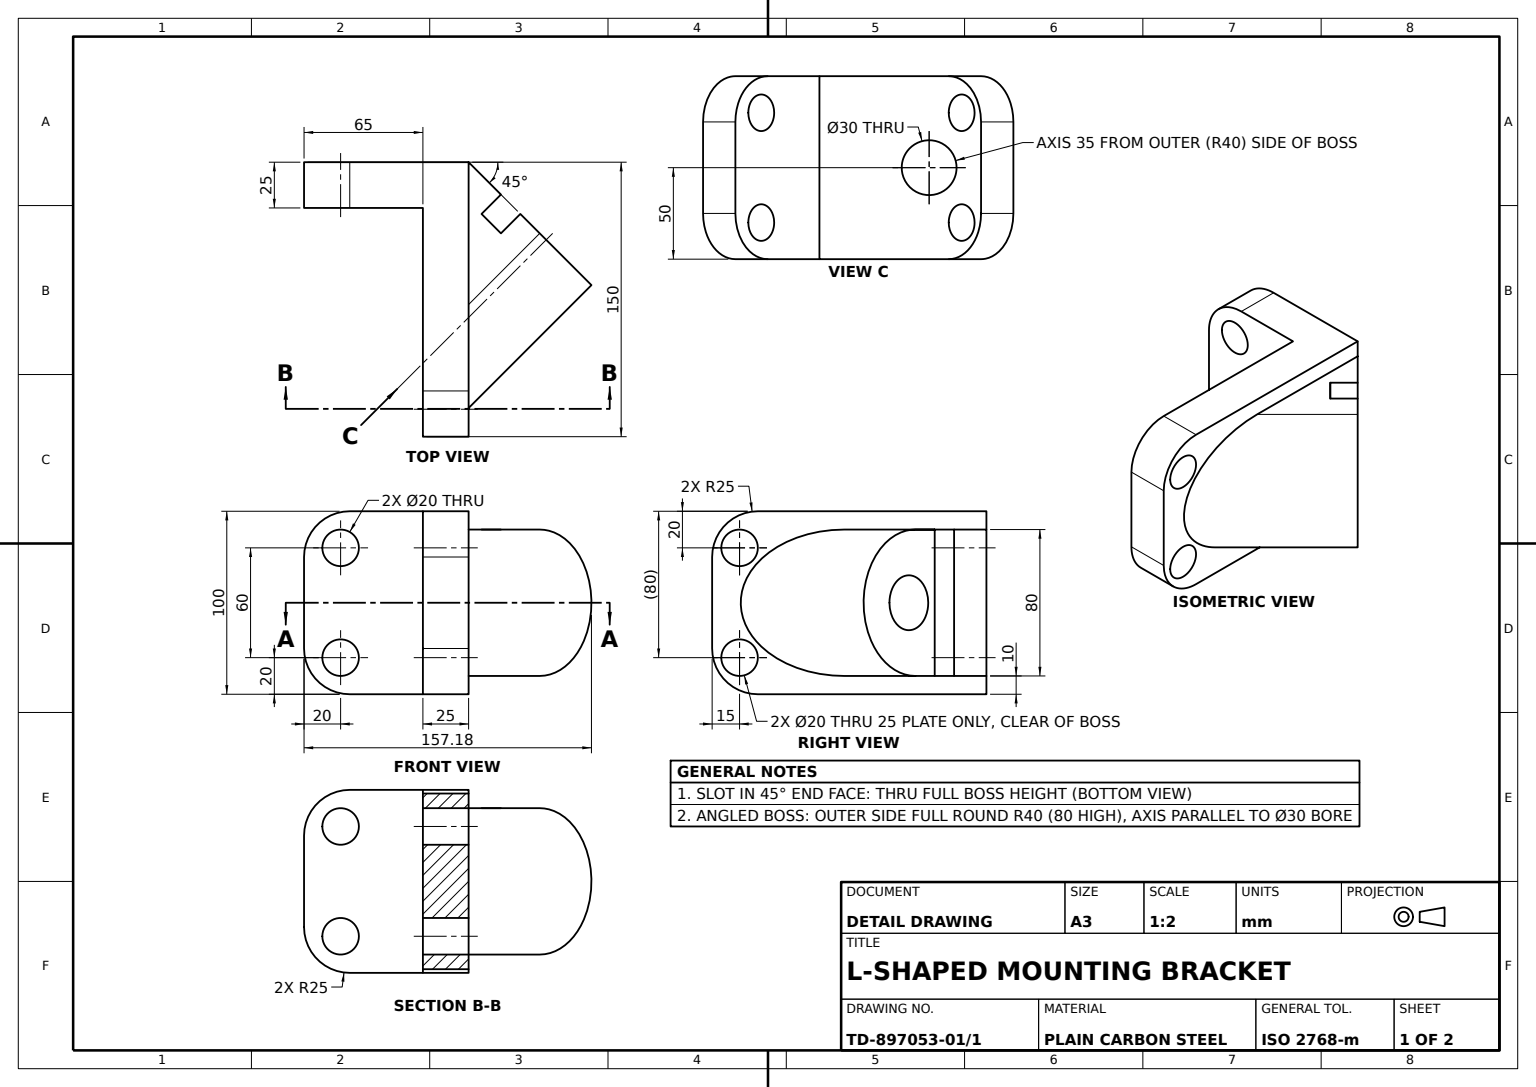
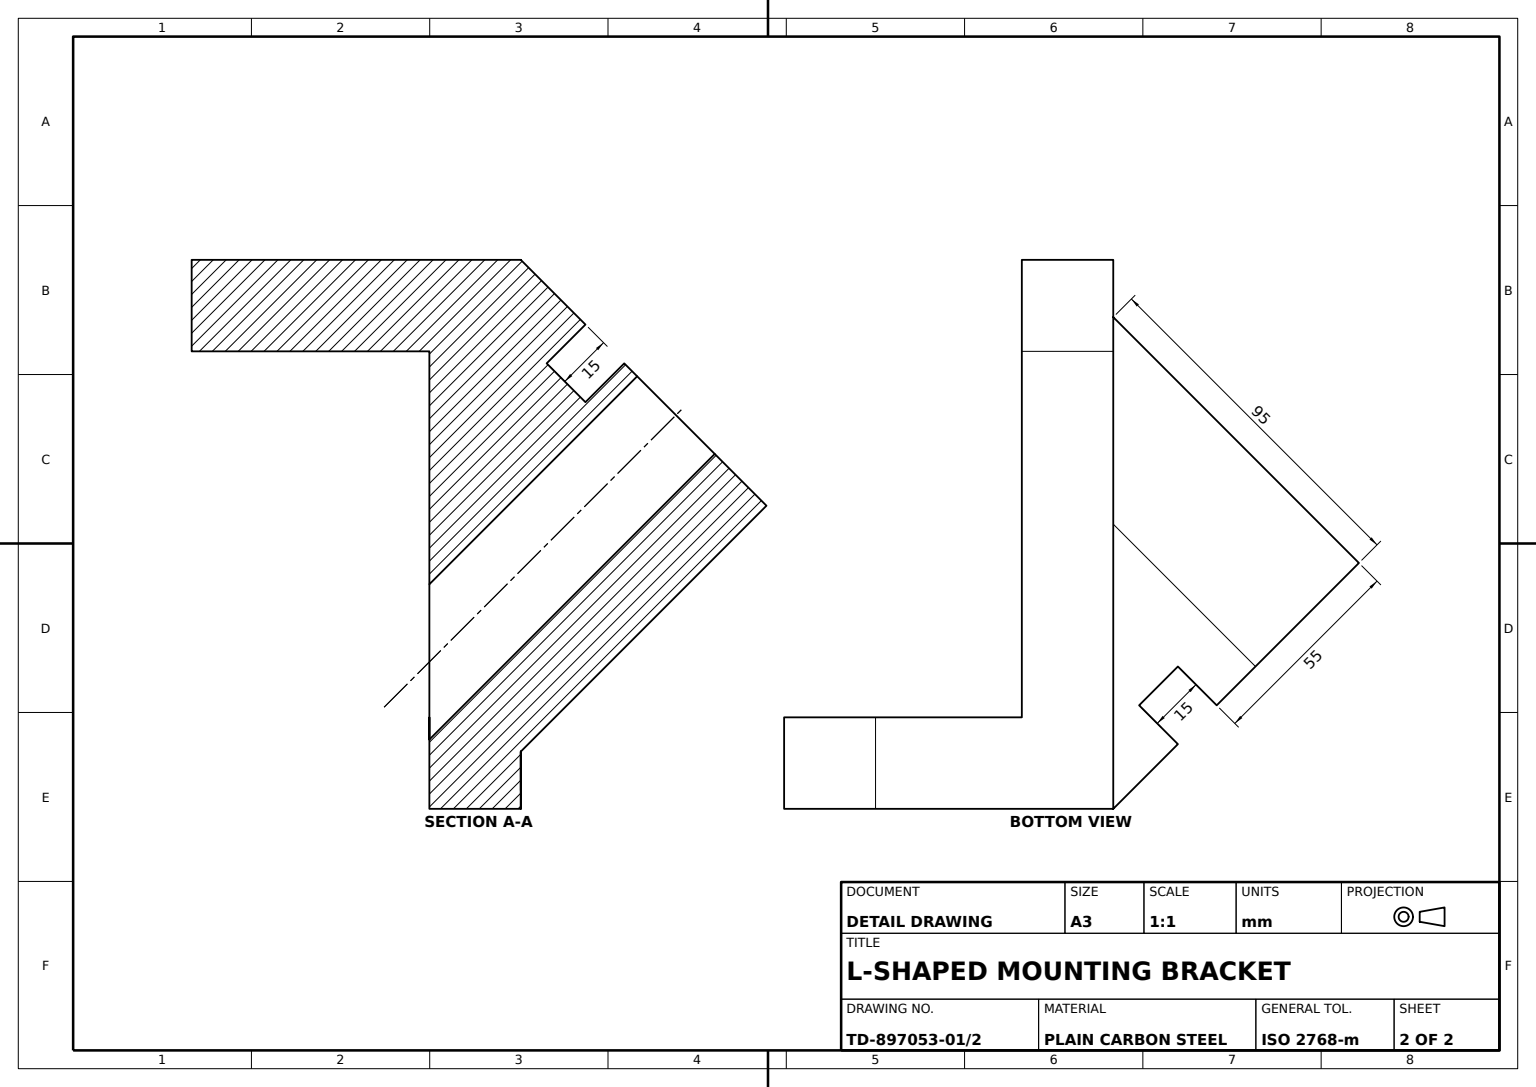
from build123d import *

# Parameters (mm, degrees)
BASE_PLATE_SKETCH_W           = 150
BASE_PLATE_SKETCH_H           = 100
BASE_PLATE_150X100X25_DEPTH   = 25
UPRIGHT_PLATE_SKETCH_W        = 25
UPRIGHT_PLATE_SKETCH_H        = 100
UPRIGHT_PLATE_DEPTH           = 65
ANGLED_BOSS_REACH             = 179.236
BOSS_SLOT_REACH               = 149.733
BOSS_BORE_REACH               = 179.236
BOSS_BORE_SKETCH_R            = 15
BASE_PLATE_HOLES_REACH        = 129.377
BASE_PLATE_HOLES_SKETCH_R     = 10
UPRIGHT_PLATE_HOLES_REACH     = 183.934
UPRIGHT_PLATE_HOLES_SKETCH_R  = 10
UPRIGHT_CORNER_FILLET_R25_A_R = 25
UPRIGHT_CORNER_FILLET_R25_B_R = 25
BASE_CORNER_FILLET_R25_A_R    = 25
BASE_CORNER_FILLET_R25_B_R    = 25


with BuildPart() as part:
    # Base Plate Sketch → Base Plate 150x100x25 (new body)
    with BuildSketch(Plane.XY):
        Rectangle(BASE_PLATE_SKETCH_W, BASE_PLATE_SKETCH_H)
    extrude(amount=BASE_PLATE_150X100X25_DEPTH)

    # Upright Plate Sketch → Upright Plate (add)
    with BuildSketch(Plane.XY.offset(25)):
        with Locations((-62.5, 0)):
            Rectangle(UPRIGHT_PLATE_SKETCH_W, UPRIGHT_PLATE_SKETCH_H)
    extrude(amount=UPRIGHT_PLATE_DEPTH)

    # Angled Boss Sketch → Angled Boss (add, up to next)
    with BuildSketch(Plane(origin=(-37.5, 0, -37.5), x_dir=(0.7071067811865512, 0, -0.7071067811865439), z_dir=(0.7071067811865439, 0, 0.7071067811865512)), mode=Mode.PRIVATE) as angled_boss_sk1:
        with BuildLine():
            Line((-53.033008589, 40), (1.966991411, 40))
            ThreePointArc((1.966991411, 40), (41.966991411, 0), (1.966991411, -40))
            Line((1.966991411, -40), (-53.033008589, -40))
            Line((-53.033008589, -40), (-53.033008589, 40))
        make_face()
    angled_boss_tool1 = extrude(angled_boss_sk1.sketch, amount=ANGLED_BOSS_REACH, mode=Mode.PRIVATE) - part.part
    add(angled_boss_tool1.solids().sort_by_distance((-44.121254, 0, -30.878746))[0])

    # Boss Slot Sketch → Boss Slot (cut, up to next)
    with BuildSketch(Plane(origin=(0, 40, 0), x_dir=(1, 0, 0), z_dir=(0, 1, 0)), mode=Mode.PRIVATE) as boss_slot_sk1:
        Polygon((-57.32233047, 17.67766953), (-46.715728753, 7.071067812), (-36.109127035, 17.67766953), (-46.715728753, 28.284271247), align=None)
    boss_slot_tool1 = extrude(boss_slot_sk1.sketch, amount=-BOSS_SLOT_REACH, mode=Mode.PRIVATE) & part.part
    add(boss_slot_tool1.solids().sort_by_distance((-46.715729, 40, -17.67767))[0], mode=Mode.SUBTRACT)

    # Boss Bore: up to this plane
    boss_bore_end = Plane(origin=(0, 0, 25), z_dir=(0, 0, -1))
    # Boss Bore Sketch → Boss Bore (cut, up to the surface)
    with BuildSketch(Plane(origin=(-37.5, 0, -37.5), x_dir=(-0.7071067811865511, 0, 0.707106781186544), z_dir=(-0.707106781186544, 0, -0.7071067811865511)), mode=Mode.PRIVATE) as boss_bore_sk1:
        with Locations((-6.966991411, 0)):
            Circle(BOSS_BORE_SKETCH_R)
    boss_bore_tool1 = split(extrude(boss_bore_sk1.sketch, amount=-BOSS_BORE_REACH, mode=Mode.PRIVATE), bisect_by=boss_bore_end, keep=Keep.BOTH, mode=Mode.PRIVATE)
    add(boss_bore_tool1.solids().sort_by_distance((-32.573593, 0, -42.426407))[0], mode=Mode.SUBTRACT)

    # Base Plate Holes Sketch → Base Plate Holes (cut, up to next)
    with BuildSketch(Plane(origin=(0, 0, 0), x_dir=(-1, 0, 0), z_dir=(0, 0, -1)), mode=Mode.PRIVATE) as base_plate_holes_sk1:
        with Locations((-60, 30)):
            Circle(BASE_PLATE_HOLES_SKETCH_R)
    base_plate_holes_tool1 = extrude(base_plate_holes_sk1.sketch, amount=-BASE_PLATE_HOLES_REACH, mode=Mode.PRIVATE) & part.part
    # Base Plate Holes Sketch → Base Plate Holes (cut, up to next)
    with BuildSketch(Plane(origin=(0, 0, 0), x_dir=(-1, 0, 0), z_dir=(0, 0, -1)), mode=Mode.PRIVATE) as base_plate_holes_sk2:
        with Locations((-60, -30)):
            Circle(BASE_PLATE_HOLES_SKETCH_R)
    base_plate_holes_tool2 = extrude(base_plate_holes_sk2.sketch, amount=-BASE_PLATE_HOLES_REACH, mode=Mode.PRIVATE) & part.part
    add(base_plate_holes_tool1.solids().sort_by_distance((60, 30, 0))[0], mode=Mode.SUBTRACT)
    add(base_plate_holes_tool2.solids().sort_by_distance((60, -30, 0))[0], mode=Mode.SUBTRACT)

    # Upright Plate Holes Sketch → Upright Plate Holes (cut, up to next)
    with BuildSketch(Plane.ZY.offset(75), mode=Mode.PRIVATE) as upright_plate_holes_sk1:
        with Locations((70, 30)):
            Circle(UPRIGHT_PLATE_HOLES_SKETCH_R)
    upright_plate_holes_tool1 = extrude(upright_plate_holes_sk1.sketch, amount=-UPRIGHT_PLATE_HOLES_REACH, mode=Mode.PRIVATE) & part.part
    # Upright Plate Holes Sketch → Upright Plate Holes (cut, up to next)
    with BuildSketch(Plane.ZY.offset(75), mode=Mode.PRIVATE) as upright_plate_holes_sk2:
        with Locations((70, -30)):
            Circle(UPRIGHT_PLATE_HOLES_SKETCH_R)
    upright_plate_holes_tool2 = extrude(upright_plate_holes_sk2.sketch, amount=-UPRIGHT_PLATE_HOLES_REACH, mode=Mode.PRIVATE) & part.part
    add(upright_plate_holes_tool1.solids().sort_by_distance((-75, 30, 70))[0], mode=Mode.SUBTRACT)
    add(upright_plate_holes_tool2.solids().sort_by_distance((-75, -30, 70))[0], mode=Mode.SUBTRACT)

    # Upright Corner Fillet R25 A
    upright_corner_fillet_r25_a_edges = [part.edges().sort_by_distance(p)[0] for p in [
        (-62.5, 50, 90),
    ]]
    fillet(upright_corner_fillet_r25_a_edges, radius=UPRIGHT_CORNER_FILLET_R25_A_R)

    # Upright Corner Fillet R25 B
    upright_corner_fillet_r25_b_edges = [part.edges().sort_by_distance(p)[0] for p in [
        (-62.5, -50, 90),
    ]]
    fillet(upright_corner_fillet_r25_b_edges, radius=UPRIGHT_CORNER_FILLET_R25_B_R)

    # Base Corner Fillet R25 A
    base_corner_fillet_r25_a_edges = [part.edges().sort_by_distance(p)[0] for p in [
        (75, -50, 12.5),
    ]]
    fillet(base_corner_fillet_r25_a_edges, radius=BASE_CORNER_FILLET_R25_A_R)

    # Base Corner Fillet R25 B
    base_corner_fillet_r25_b_edges = [part.edges().sort_by_distance(p)[0] for p in [
        (75, 50, 12.5),
    ]]
    fillet(base_corner_fillet_r25_b_edges, radius=BASE_CORNER_FILLET_R25_B_R)


solid = part.part
